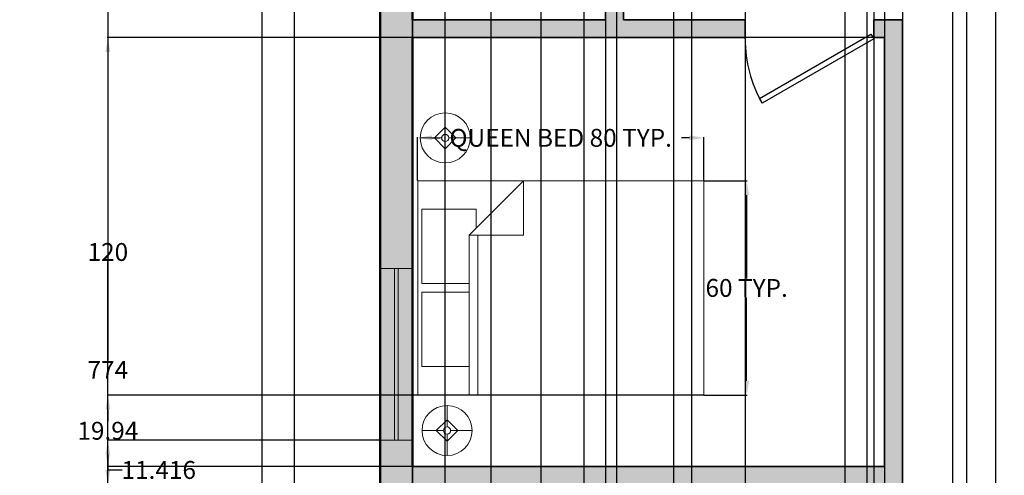
# Model space of a CAD drawing. Units: inches. Extents: x 882 to 1363, y 890 to 1847.
# Tile 5 of 9: x 882 to 1157, y 1351 to 1479. Entities that reach past the tile are written whole.
import ezdxf

# ---------------------------------------------------------------- set-up
doc = ezdxf.new("R2010")
doc.units = ezdxf.units.IN
doc.header["$MEASUREMENT"] = 0
for name, color, linetype, lineweight in [('A-ANNO-DIMS', 2, 'Continuous', 18), ('C-PROP', 7, 'Continuous', 25), ('doors', 3, 'Continuous', 25), ('furniture', 10, 'Continuous', 18), ('inner wall', 50, 'Continuous', 35), ('outer wall', 40, 'Continuous', 50), ('windows', 226, 'Continuous', 18)]:
    doc.layers.add(name, color=color, linetype=linetype, lineweight=lineweight)
doc.layers.add('A-WALL-PATT', color=251, linetype='Continuous', lineweight=13, true_color=0x636466)
doc.styles.get("Standard").update_dxf_attribs({"font": 'arial.ttf'})
doc.dimstyles.get("Standard").update_dxf_attribs({"dimtxt": 5, "dimasz": 4, "dimexe": 0.18, "dimexo": 0.0625, "dimgap": 0.09, "dimtad": 0, "dimtih": 1, "dimtoh": 1, "dimdec": 1, "dimzin": 0, "dimdsep": 46, "dimlunit": 3, "dimtxsty": 'Standard', "dimcen": 0.09, "dimadec": 0, "dimazin": 0, "dimtfac": 1, "dimtdec": 1, "dimtofl": 0, "dimtmove": 0, "dimatfit": 3, "dimfxl": 1, "dimtolj": 1, "dimtzin": 0, "dimarcsym": 0})

# ---------------------------------------------------------------- blocks, each defined once
blk = doc.blocks.new('*U2')
for p, q in [((0, 0), (0, -6)), ((40, 0), (40, -6))]:
    blk.add_line(p, q)
blk.add_lwpolyline([(0, 0), (34.64, 20), (35.52, 18.48), (0.87, -1.52)], close=True)
blk.add_arc((0, 0), 40, 0, 30)
blk = doc.blocks.new('Bed - Queen')
for p, q in [((0, -80.00003), (0, 0)), ((0, 0), (59.99999, 0)), ((59.99999, 0), (59.99999, -80.00003)), ((7.99999, -1.2), (28.79998, -1.2)), ((7.99999, -14.4), (7.99999, -1.2)), ((28.79998, -1.2), (28.79998, -14.4)), ((31.19999, -1.2), (51.99999, -1.2)), ((31.19999, -14.4), (31.19999, -1.2)), ((51.99999, -1.2), (51.99999, -16.4)), ((0, -14.4), (44.8, -14.4)), ((59.99999, -29.6), (44.8, -14.4)), ((44.8, -14.4), (44.8, -29.6)), ((51.99999, -16.4), (46.79936, -16.4)), ((44.8, -16.8), (0, -16.8)), ((44.8, -29.6), (59.99999, -29.6)), ((59.99999, -80.00003), (0, -80.00003))]:
    blk.add_line(p, q)
blk = doc.blocks.new('Lamp - Table')
for p, q in [((0, 7), (0, 1)), ((0, 3), (-3, 0)), ((3, 0), (0, 3)), ((-1, 0), (-7, 0)), ((-3, 0), (0, -3)), ((0, -3), (3, 0)), ((1, 0), (7, 0)), ((0, -1), (0, -7))]:
    blk.add_line(p, q)
for radius in [7, 1]:
    blk.add_circle((0, 0), radius)
blk = doc.blocks.new('WIN-48IN-9IN')
for p, q in [((4, 0), (4, 48)), ((5, 0), (5, 48))]:
    blk.add_line(p, q)
blk.add_lwpolyline([(0, 48), (9, 48), (9, 0), (0, 0)], close=True)
blk = doc.blocks.new('*D23')
at = {"layer": 'A-ANNO-DIMS', "color": 0, "lineweight": -2, "transparency": 16777216}
for p, q in [((993.28, 1433.75), (993.28, 1445.87)), ((997.28, 1445.69), (999.49, 1445.69)), ((1069.28, 1445.69), (1067.08, 1445.69)), ((1073.28, 1433.75), (1073.28, 1445.87))]:
    blk.add_line(p, q, dxfattribs=at)
at = {"layer": 'A-ANNO-DIMS', "color": 0, "transparency": 16777216}
for points in [[(997.28, 1446.35), (997.28, 1445.02), (993.28, 1445.69)], [(1069.28, 1446.35), (1069.28, 1445.02), (1073.28, 1445.69)]]:
    blk.add_solid(points, dxfattribs=at)
at = {"layer": 'Defpoints', "color": 0, "transparency": 16777216}
for p in [(993.28, 1445.69), (993.28, 1433.69), (1073.28, 1433.69)]:
    blk.add_point(p, dxfattribs=at)
at = {"layer": 'A-ANNO-DIMS', "color": 0, "transparency": 16777216, "insert": (1033.28, 1445.69), "char_height": 5, "attachment_point": 5}
blk.add_mtext('\\A1;QUEEN BED 80 TYP.', dxfattribs=at)
blk = doc.blocks.new('*D24')
at = {"layer": 'A-ANNO-DIMS', "color": 0, "lineweight": -2, "transparency": 16777216}
for p, q in [((1073.34, 1433.69), (1085.46, 1433.69)), ((1085.28, 1429.69), (1085.28, 1406.33)), ((1085.28, 1377.69), (1085.28, 1401.04)), ((1073.34, 1373.69), (1085.46, 1373.69))]:
    blk.add_line(p, q, dxfattribs=at)
at = {"layer": 'A-ANNO-DIMS', "color": 0, "transparency": 16777216}
for points in [[(1084.61, 1429.69), (1085.95, 1429.69), (1085.28, 1433.69)], [(1084.61, 1377.69), (1085.95, 1377.69), (1085.28, 1373.69)]]:
    blk.add_solid(points, dxfattribs=at)
at = {"layer": 'Defpoints', "color": 0, "transparency": 16777216}
for p in [(1073.28, 1433.69), (1085.28, 1433.69), (1073.28, 1373.69)]:
    blk.add_point(p, dxfattribs=at)
at = {"layer": 'A-ANNO-DIMS', "color": 0, "transparency": 16777216, "insert": (1085.28, 1403.69), "char_height": 5, "attachment_point": 5}
blk.add_mtext('\\A1;60 TYP.', dxfattribs=at)
blk = doc.blocks.new('*D37')
at = {"layer": 'A-ANNO-DIMS', "color": 0, "lineweight": -2, "transparency": 16777216}
for p, q in [((982.78, 1767.75), (906.46, 1767.75)), ((906.64, 1763.75), (906.64, 1383.34)), ((906.64, 997.75), (906.64, 1378.16)), ((982.78, 993.75), (906.46, 993.75))]:
    blk.add_line(p, q, dxfattribs=at)
at = {"layer": 'A-ANNO-DIMS', "color": 0, "transparency": 16777216}
for points in [[(905.97, 1763.75), (907.3, 1763.75), (906.64, 1767.75)], [(905.97, 997.75), (907.3, 997.75), (906.64, 993.75)]]:
    blk.add_solid(points, dxfattribs=at)
at = {"layer": 'Defpoints', "color": 0, "transparency": 16777216}
for p in [(906.64, 1767.75), (982.84, 1767.75), (982.84, 993.75)]:
    blk.add_point(p, dxfattribs=at)
at = {"layer": 'A-ANNO-DIMS', "color": 0, "transparency": 16777216, "insert": (906.64, 1380.75), "char_height": 5, "attachment_point": 5}
blk.add_mtext('\\A1;774', dxfattribs=at)
blk = doc.blocks.new('*D40')
at = {"layer": 'A-ANNO-DIMS', "color": 0, "lineweight": -2, "transparency": 16777216}
for p, q in [((991.84, 1758.69), (991.84, 893.37)), ((1064.84, 1758.69), (1064.84, 893.37)), ((995.84, 893.55), (1024.69, 893.55)), ((1060.84, 893.55), (1031.99, 893.55))]:
    blk.add_line(p, q, dxfattribs=at)
at = {"layer": 'A-ANNO-DIMS', "color": 0, "transparency": 16777216}
for points in [[(995.84, 894.21), (995.84, 892.88), (991.84, 893.55)], [(1060.84, 894.21), (1060.84, 892.88), (1064.84, 893.55)]]:
    blk.add_solid(points, dxfattribs=at)
at = {"layer": 'Defpoints', "color": 0, "transparency": 16777216}
for p in [(991.84, 1758.75), (1064.84, 1758.75), (1064.84, 893.55)]:
    blk.add_point(p, dxfattribs=at)
at = {"layer": 'A-ANNO-DIMS', "color": 0, "transparency": 16777216, "insert": (1028.34, 893.55), "char_height": 5, "attachment_point": 5}
blk.add_mtext('\\A1;73', dxfattribs=at)
blk = doc.blocks.new('*D41')
at = {"layer": 'A-ANNO-DIMS', "color": 0, "lineweight": -2, "transparency": 16777216}
for p, q in [((1069.84, 1758.69), (1069.84, 893.37)), ((1154.84, 1758.69), (1154.84, 893.37)), ((1073.84, 893.55), (1108.65, 893.55)), ((1150.84, 893.55), (1116.03, 893.55))]:
    blk.add_line(p, q, dxfattribs=at)
at = {"layer": 'A-ANNO-DIMS', "color": 0, "transparency": 16777216}
for points in [[(1073.84, 894.21), (1073.84, 892.88), (1069.84, 893.55)], [(1150.84, 894.21), (1150.84, 892.88), (1154.84, 893.55)]]:
    blk.add_solid(points, dxfattribs=at)
at = {"layer": 'Defpoints', "color": 0, "transparency": 16777216}
for p in [(1069.84, 1758.75), (1154.84, 1758.75), (1154.84, 893.55)]:
    blk.add_point(p, dxfattribs=at)
at = {"layer": 'A-ANNO-DIMS', "color": 0, "transparency": 16777216, "insert": (1112.34, 893.55), "char_height": 5, "attachment_point": 5}
blk.add_mtext('\\A1;85', dxfattribs=at)
blk = doc.blocks.new('*D47')
at = {"layer": 'A-ANNO-DIMS', "color": 0, "lineweight": -2, "transparency": 16777216}
for p, q in [((1123.84, 1567.69), (1123.84, 893.37)), ((1128.84, 1567.69), (1128.84, 893.37)), ((1119.84, 893.55), (1115.84, 893.55)), ((1132.84, 893.55), (1136.84, 893.55))]:
    blk.add_line(p, q, dxfattribs=at)
at = {"layer": 'A-ANNO-DIMS', "color": 0, "transparency": 16777216}
for points in [[(1119.84, 894.21), (1119.84, 892.88), (1123.84, 893.55)], [(1132.84, 894.21), (1132.84, 892.88), (1128.84, 893.55)]]:
    blk.add_solid(points, dxfattribs=at)
at = {"layer": 'Defpoints', "color": 0, "transparency": 16777216}
for p in [(1123.84, 1567.75), (1128.84, 1567.75), (1128.84, 893.55)]:
    blk.add_point(p, dxfattribs=at)
at = {"layer": 'A-ANNO-DIMS', "color": 0, "transparency": 16777216, "insert": (1126.34, 893.55), "char_height": 5, "attachment_point": 5}
blk.add_mtext('\\A1;5', dxfattribs=at)
blk = doc.blocks.new('*D48')
at = {"layer": 'A-ANNO-DIMS', "color": 0, "lineweight": -2, "transparency": 16777216}
for p, q in [((1084.84, 1562.69), (1084.84, 893.37)), ((1120.84, 1562.69), (1120.84, 893.37)), ((1088.84, 893.55), (1099.17, 893.55)), ((1116.84, 893.55), (1106.51, 893.55))]:
    blk.add_line(p, q, dxfattribs=at)
at = {"layer": 'A-ANNO-DIMS', "color": 0, "transparency": 16777216}
for points in [[(1088.84, 894.21), (1088.84, 892.88), (1084.84, 893.55)], [(1116.84, 894.21), (1116.84, 892.88), (1120.84, 893.55)]]:
    blk.add_solid(points, dxfattribs=at)
at = {"layer": 'Defpoints', "color": 0, "transparency": 16777216}
for p in [(1084.84, 1562.75), (1120.84, 1562.75), (1120.84, 893.55)]:
    blk.add_point(p, dxfattribs=at)
at = {"layer": 'A-ANNO-DIMS', "color": 0, "transparency": 16777216, "insert": (1102.84, 893.55), "char_height": 5, "attachment_point": 5}
blk.add_mtext('\\A1;36', dxfattribs=at)
blk = doc.blocks.new('*D51')
at = {"layer": 'A-ANNO-DIMS', "color": 0, "lineweight": -2, "transparency": 16777216}
for p, q in [((982.84, 1767.69), (982.84, 893.37)), ((1000.84, 1767.69), (1000.84, 893.37)), ((986.84, 893.55), (996.84, 893.55)), ((1000.84, 893.55), (1004.84, 893.55))]:
    blk.add_line(p, q, dxfattribs=at)
at = {"layer": 'A-ANNO-DIMS', "color": 0, "transparency": 16777216}
for points in [[(986.84, 894.21), (986.84, 892.88), (982.84, 893.55)], [(996.84, 894.21), (996.84, 892.88), (1000.84, 893.55)]]:
    blk.add_solid(points, dxfattribs=at)
at = {"layer": 'Defpoints', "color": 0, "transparency": 16777216}
for p in [(982.84, 1767.75), (1000.84, 1767.75), (1000.84, 893.55)]:
    blk.add_point(p, dxfattribs=at)
at = {"layer": 'A-ANNO-DIMS', "color": 0, "transparency": 16777216, "insert": (1015.08, 893.55), "char_height": 5, "attachment_point": 5}
blk.add_mtext('\\A1;18.006', dxfattribs=at)
blk = doc.blocks.new('*D52')
at = {"layer": 'A-ANNO-DIMS', "color": 0, "lineweight": -2, "transparency": 16777216}
for p, q in [((1048.84, 1767.69), (1048.84, 893.37)), ((1118.86, 1767.69), (1118.86, 893.37)), ((1052.84, 893.55), (1075.83, 893.55)), ((1114.86, 893.55), (1091.87, 893.55))]:
    blk.add_line(p, q, dxfattribs=at)
at = {"layer": 'A-ANNO-DIMS', "color": 0, "transparency": 16777216}
for points in [[(1052.84, 894.21), (1052.84, 892.88), (1048.84, 893.55)], [(1114.86, 894.21), (1114.86, 892.88), (1118.86, 893.55)]]:
    blk.add_solid(points, dxfattribs=at)
at = {"layer": 'Defpoints', "color": 0, "transparency": 16777216}
for p in [(1048.84, 1767.75), (1118.86, 1767.75), (1118.86, 893.55)]:
    blk.add_point(p, dxfattribs=at)
at = {"layer": 'A-ANNO-DIMS', "color": 0, "transparency": 16777216, "insert": (1083.85, 893.55), "char_height": 5, "attachment_point": 5}
blk.add_mtext('\\A1;70.01', dxfattribs=at)
blk = doc.blocks.new('*D53')
at = {"layer": 'A-ANNO-DIMS', "color": 0, "lineweight": -2, "transparency": 16777216}
for p, q in [((1142.86, 1767.69), (1142.86, 893.37)), ((1171.41, 1767.69), (1171.41, 893.37)), ((1138.86, 893.55), (1134.86, 893.55)), ((1175.41, 893.55), (1179.41, 893.55))]:
    blk.add_line(p, q, dxfattribs=at)
at = {"layer": 'A-ANNO-DIMS', "color": 0, "transparency": 16777216}
for points in [[(1138.86, 894.21), (1138.86, 892.88), (1142.86, 893.55)], [(1175.41, 894.21), (1175.41, 892.88), (1171.41, 893.55)]]:
    blk.add_solid(points, dxfattribs=at)
at = {"layer": 'Defpoints', "color": 0, "transparency": 16777216}
for p in [(1142.86, 1767.75), (1171.41, 1767.75), (1171.41, 893.55)]:
    blk.add_point(p, dxfattribs=at)
at = {"layer": 'A-ANNO-DIMS', "color": 0, "transparency": 16777216, "insert": (1157.14, 893.55), "char_height": 5, "attachment_point": 5}
blk.add_mtext('\\A1;28.554', dxfattribs=at)
blk = doc.blocks.new('*D58')
at = {"layer": 'A-ANNO-DIMS', "color": 0, "lineweight": -2, "transparency": 16777216}
for p, q in [((1123.78, 1473.75), (906.46, 1473.75)), ((906.64, 1469.75), (906.64, 1416.39)), ((906.64, 1357.75), (906.64, 1411.11)), ((1123.78, 1353.75), (906.46, 1353.75))]:
    blk.add_line(p, q, dxfattribs=at)
at = {"layer": 'A-ANNO-DIMS', "color": 0, "transparency": 16777216}
for points in [[(905.97, 1469.75), (907.3, 1469.75), (906.64, 1473.75)], [(905.97, 1357.75), (907.3, 1357.75), (906.64, 1353.75)]]:
    blk.add_solid(points, dxfattribs=at)
at = {"layer": 'Defpoints', "color": 0, "transparency": 16777216}
for p in [(1123.84, 1473.75), (906.64, 1353.75), (1123.84, 1353.75)]:
    blk.add_point(p, dxfattribs=at)
at = {"layer": 'A-ANNO-DIMS', "color": 0, "transparency": 16777216, "insert": (906.64, 1413.75), "char_height": 5, "attachment_point": 5}
blk.add_mtext('\\A1;120', dxfattribs=at)
blk = doc.blocks.new('*D59')
at = {"layer": 'A-ANNO-DIMS', "color": 0, "lineweight": -2, "transparency": 16777216}
for p, q in [((982.78, 1361.08), (906.46, 1361.08)), ((906.64, 1357.08), (906.64, 1352.75)), ((991.78, 1348.75), (906.46, 1348.75)), ((906.64, 1348.75), (906.64, 1344.75)), ((906.64, 1344.75), (902.64, 1344.75))]:
    blk.add_line(p, q, dxfattribs=at)
at = {"layer": 'A-ANNO-DIMS', "color": 0, "transparency": 16777216}
for points in [[(905.97, 1357.08), (907.3, 1357.08), (906.64, 1361.08)], [(905.97, 1352.75), (907.3, 1352.75), (906.64, 1348.75)]]:
    blk.add_solid(points, dxfattribs=at)
at = {"layer": 'Defpoints', "color": 0, "transparency": 16777216}
for p in [(982.84, 1361.08), (906.64, 1348.75), (991.84, 1348.75)]:
    blk.add_point(p, dxfattribs=at)
at = {"layer": 'A-ANNO-DIMS', "color": 0, "transparency": 16777216, "insert": (892.4, 1344.75), "char_height": 5, "attachment_point": 5}
blk.add_mtext('\\A1;12.328', dxfattribs=at)
blk = doc.blocks.new('*D68')
at = {"layer": 'A-ANNO-DIMS', "color": 0, "lineweight": -2, "transparency": 16777216}
for p, q in [((1027.84, 1142.81), (1027.84, 1844.13)), ((1031.84, 1843.95), (1066.65, 1843.95)), ((1108.84, 1843.95), (1074.03, 1843.95)), ((1112.84, 1142.81), (1112.84, 1844.13))]:
    blk.add_line(p, q, dxfattribs=at)
at = {"layer": 'A-ANNO-DIMS', "color": 0, "transparency": 16777216}
for points in [[(1031.84, 1844.62), (1031.84, 1843.29), (1027.84, 1843.95)], [(1108.84, 1844.62), (1108.84, 1843.29), (1112.84, 1843.95)]]:
    blk.add_solid(points, dxfattribs=at)
at = {"layer": 'Defpoints', "color": 0, "transparency": 16777216}
for p in [(1112.84, 1843.95), (1027.84, 1142.75), (1112.84, 1142.75)]:
    blk.add_point(p, dxfattribs=at)
at = {"layer": 'A-ANNO-DIMS', "color": 0, "transparency": 16777216, "insert": (1070.34, 1843.95), "char_height": 5, "attachment_point": 5}
blk.add_mtext('\\A1;85', dxfattribs=at)
blk = doc.blocks.new('*D74')
at = {"layer": 'A-ANNO-DIMS', "color": 0, "lineweight": -2, "transparency": 16777216}
for p, q in [((991.84, 1002.81), (991.84, 1844.13)), ((995.84, 1843.95), (1012.06, 1843.95)), ((1035.84, 1843.95), (1019.62, 1843.95)), ((1039.84, 1002.81), (1039.84, 1844.13))]:
    blk.add_line(p, q, dxfattribs=at)
at = {"layer": 'A-ANNO-DIMS', "color": 0, "transparency": 16777216}
for points in [[(995.84, 1844.62), (995.84, 1843.29), (991.84, 1843.95)], [(1035.84, 1844.62), (1035.84, 1843.29), (1039.84, 1843.95)]]:
    blk.add_solid(points, dxfattribs=at)
at = {"layer": 'Defpoints', "color": 0, "transparency": 16777216}
for p in [(1039.84, 1843.95), (991.84, 1002.75), (1039.84, 1002.75)]:
    blk.add_point(p, dxfattribs=at)
at = {"layer": 'A-ANNO-DIMS', "color": 0, "transparency": 16777216, "insert": (1015.84, 1843.95), "char_height": 5, "attachment_point": 5}
blk.add_mtext('\\A1;48', dxfattribs=at)
blk = doc.blocks.new('*D78')
at = {"layer": 'A-ANNO-DIMS', "color": 0, "lineweight": -2, "transparency": 16777216}
for p, q in [((1146.84, 1274.81), (1146.84, 1844.13)), ((1150.84, 1843.95), (1179.69, 1843.95)), ((1215.84, 1843.95), (1186.99, 1843.95)), ((1219.84, 1274.81), (1219.84, 1844.13))]:
    blk.add_line(p, q, dxfattribs=at)
at = {"layer": 'A-ANNO-DIMS', "color": 0, "transparency": 16777216}
for points in [[(1150.84, 1844.62), (1150.84, 1843.29), (1146.84, 1843.95)], [(1215.84, 1844.62), (1215.84, 1843.29), (1219.84, 1843.95)]]:
    blk.add_solid(points, dxfattribs=at)
at = {"layer": 'Defpoints', "color": 0, "transparency": 16777216}
for p in [(1219.84, 1843.95), (1146.84, 1274.75), (1219.84, 1274.75)]:
    blk.add_point(p, dxfattribs=at)
at = {"layer": 'A-ANNO-DIMS', "color": 0, "transparency": 16777216, "insert": (1183.34, 1843.95), "char_height": 5, "attachment_point": 5}
blk.add_mtext('\\A1;73', dxfattribs=at)
blk = doc.blocks.new('*D83')
at = {"layer": 'A-ANNO-DIMS', "color": 0, "lineweight": -2, "transparency": 16777216}
for p, q in [((906.64, 1348.75), (906.64, 1352.75)), ((906.64, 1352.75), (910.64, 1352.75)), ((991.78, 1348.75), (906.46, 1348.75)), ((906.64, 1341.33), (906.64, 1344.75)), ((982.78, 1337.33), (906.46, 1337.33))]:
    blk.add_line(p, q, dxfattribs=at)
at = {"layer": 'A-ANNO-DIMS', "color": 0, "transparency": 16777216}
for points in [[(905.97, 1344.75), (907.3, 1344.75), (906.64, 1348.75)], [(905.97, 1341.33), (907.3, 1341.33), (906.64, 1337.33)]]:
    blk.add_solid(points, dxfattribs=at)
at = {"layer": 'Defpoints', "color": 0, "transparency": 16777216}
for p in [(906.64, 1348.75), (991.84, 1348.75), (982.84, 1337.33)]:
    blk.add_point(p, dxfattribs=at)
at = {"layer": 'A-ANNO-DIMS', "color": 0, "transparency": 16777216, "insert": (920.87, 1352.75), "char_height": 5, "attachment_point": 5}
blk.add_mtext('\\A1;11.416', dxfattribs=at)
blk = doc.blocks.new('*D85')
at = {"layer": 'A-ANNO-DIMS', "color": 0, "lineweight": -2, "transparency": 16777216}
for p, q in [((1045.84, 1562.69), (1045.84, 893.37)), ((1084.84, 1562.69), (1084.84, 893.37)), ((1049.84, 893.55), (1061.66, 893.55)), ((1080.84, 893.55), (1069.01, 893.55))]:
    blk.add_line(p, q, dxfattribs=at)
at = {"layer": 'A-ANNO-DIMS', "color": 0, "transparency": 16777216}
for points in [[(1049.84, 894.21), (1049.84, 892.88), (1045.84, 893.55)], [(1080.84, 894.21), (1080.84, 892.88), (1084.84, 893.55)]]:
    blk.add_solid(points, dxfattribs=at)
at = {"layer": 'Defpoints', "color": 0, "transparency": 16777216}
for p in [(1045.84, 1562.75), (1084.84, 1562.75), (1084.84, 893.55)]:
    blk.add_point(p, dxfattribs=at)
at = {"layer": 'A-ANNO-DIMS', "color": 0, "transparency": 16777216, "insert": (1065.34, 893.55), "char_height": 5, "attachment_point": 5}
blk.add_mtext('\\A1;39', dxfattribs=at)
blk = doc.blocks.new('*D88')
at = {"layer": 'A-ANNO-DIMS', "color": 0, "lineweight": -2, "transparency": 16777216}
for p, q in [((1128.84, 1567.69), (1128.84, 893.37)), ((1211.84, 1562.69), (1211.84, 893.37)), ((1132.84, 893.55), (1166.66, 893.55)), ((1207.84, 893.55), (1174.01, 893.55))]:
    blk.add_line(p, q, dxfattribs=at)
at = {"layer": 'A-ANNO-DIMS', "color": 0, "transparency": 16777216}
for points in [[(1132.84, 894.21), (1132.84, 892.88), (1128.84, 893.55)], [(1207.84, 894.21), (1207.84, 892.88), (1211.84, 893.55)]]:
    blk.add_solid(points, dxfattribs=at)
at = {"layer": 'Defpoints', "color": 0, "transparency": 16777216}
for p in [(1128.84, 1567.75), (1211.84, 1562.75), (1211.84, 893.55)]:
    blk.add_point(p, dxfattribs=at)
at = {"layer": 'A-ANNO-DIMS', "color": 0, "transparency": 16777216, "insert": (1170.34, 893.55), "char_height": 5, "attachment_point": 5}
blk.add_mtext('\\A1;83', dxfattribs=at)
blk = doc.blocks.new('*D89')
at = {"layer": 'A-ANNO-DIMS', "color": 0, "lineweight": -2, "transparency": 16777216}
for p, q in [((991.84, 1473.69), (991.84, 893.37)), ((1084.84, 1473.69), (1084.84, 893.37)), ((995.84, 893.55), (1034.67, 893.55)), ((1080.84, 893.55), (1042.01, 893.55))]:
    blk.add_line(p, q, dxfattribs=at)
at = {"layer": 'A-ANNO-DIMS', "color": 0, "transparency": 16777216}
for points in [[(995.84, 894.21), (995.84, 892.88), (991.84, 893.55)], [(1080.84, 894.21), (1080.84, 892.88), (1084.84, 893.55)]]:
    blk.add_solid(points, dxfattribs=at)
at = {"layer": 'Defpoints', "color": 0, "transparency": 16777216}
for p in [(991.84, 1473.75), (1084.84, 1473.75), (1084.84, 893.55)]:
    blk.add_point(p, dxfattribs=at)
at = {"layer": 'A-ANNO-DIMS', "color": 0, "transparency": 16777216, "insert": (1038.34, 893.55), "char_height": 5, "attachment_point": 5}
blk.add_mtext('\\A1;93', dxfattribs=at)
blk = doc.blocks.new('*D92')
at = {"layer": 'A-ANNO-DIMS', "color": 0, "lineweight": -2, "transparency": 16777216}
for p, q in [((1073.22, 1373.69), (906.46, 1373.69)), ((906.64, 1369.69), (906.64, 1366.36)), ((906.64, 1357.75), (906.64, 1361.08)), ((1123.78, 1353.75), (906.46, 1353.75))]:
    blk.add_line(p, q, dxfattribs=at)
at = {"layer": 'A-ANNO-DIMS', "color": 0, "transparency": 16777216}
for points in [[(905.97, 1369.69), (907.3, 1369.69), (906.64, 1373.69)], [(905.97, 1357.75), (907.3, 1357.75), (906.64, 1353.75)]]:
    blk.add_solid(points, dxfattribs=at)
at = {"layer": 'Defpoints', "color": 0, "transparency": 16777216}
for p in [(1073.28, 1373.69), (906.64, 1353.75), (1123.84, 1353.75)]:
    blk.add_point(p, dxfattribs=at)
at = {"layer": 'A-ANNO-DIMS', "color": 0, "transparency": 16777216, "insert": (906.64, 1363.72), "char_height": 5, "attachment_point": 5}
blk.add_mtext('\\A1;19.94', dxfattribs=at)
blk = doc.blocks.new('*D93')
at = {"layer": 'A-ANNO-DIMS', "color": 0, "lineweight": -2, "transparency": 16777216}
for p, q in [((987.84, 1843.95), (983.84, 1843.95)), ((991.84, 1337.4), (991.84, 1844.13)), ((1013.79, 1306.45), (1013.79, 1844.13)), ((1017.79, 1843.95), (1021.79, 1843.95))]:
    blk.add_line(p, q, dxfattribs=at)
at = {"layer": 'A-ANNO-DIMS', "color": 0, "transparency": 16777216}
for points in [[(987.84, 1844.62), (987.84, 1843.29), (991.84, 1843.95)], [(1017.79, 1844.62), (1017.79, 1843.29), (1013.79, 1843.95)]]:
    blk.add_solid(points, dxfattribs=at)
at = {"layer": 'Defpoints', "color": 0, "transparency": 16777216}
for p in [(1013.79, 1843.95), (991.84, 1337.33), (1013.79, 1306.39)]:
    blk.add_point(p, dxfattribs=at)
at = {"layer": 'A-ANNO-DIMS', "color": 0, "transparency": 16777216, "insert": (1002.81, 1843.95), "char_height": 5, "attachment_point": 5}
blk.add_mtext('\\A1;21.95', dxfattribs=at)

msp = doc.modelspace()

# ---------------------------------------------------------------- hatches: boundary and pattern name
at = {"layer": 'A-WALL-PATT'}
h = msp.add_hatch(color=256, dxfattribs=at)
h.dxf.hatch_style = 1
h.paths.add_polyline_path([(1050.8388, 1481.7495), (1050.8388, 1478.7495), (1084.8388, 1478.7495), (1084.8388, 1473.7495), (991.8388, 1473.7495), (991.8388, 1361.0778), (982.8388, 1361.0778), (982.8388, 1556.1531), (991.8388, 1556.1531), (991.8388, 1478.7495), (1045.8388, 1478.7495), (1045.8388, 1481.7479), (1045.4161, 1481.7477), (1030.9055, 1506.8563), (1032.004, 1507.4911), (1046.5146, 1482.3825), (1045.4161, 1481.7477), (1045.8388, 1481.7479), (1045.8388, 1481.7495)])
h.paths.add_polyline_path([(1128.8388, 1478.7495), (1120.8388, 1478.7495), (1120.8388, 1473.7495), (1123.8388, 1473.7495), (1123.8388, 1353.7495), (991.8388, 1353.7495), (991.8388, 1361.0778), (982.8388, 1361.0778), (982.8388, 1337.3333), (991.8388, 1337.3333), (991.8388, 1348.7495), (1128.8388, 1348.7495)])
h.paths.add_polyline_path([(1118.8585, 1767.7495), (1048.8447, 1767.7495), (1048.8447, 1758.7495), (1064.8388, 1758.7495), (1069.8388, 1758.7495), (1118.8585, 1758.7495)])
h.paths.add_polyline_path([(1171.4129, 1767.7495), (1142.8585, 1767.7495), (1142.8585, 1758.7495), (1154.8388, 1758.7495), (1154.8388, 1710.7495), (1069.8388, 1710.7495), (1069.8388, 1713.7495), (1064.8388, 1713.7495), (1064.8388, 1705.7495), (1123.8388, 1705.7495), (1123.8388, 1567.7495), (1120.8388, 1567.7495), (1120.8388, 1562.7495), (1123.8388, 1562.7495), (1211.8388, 1562.7495), (1211.8388, 1567.7495), (1128.8388, 1567.7495), (1128.8388, 1705.7495), (1211.8388, 1705.7495), (1211.8388, 1710.7495), (1159.8388, 1710.7495), (1159.8388, 1758.7495), (1171.4129, 1758.7495)])
h.paths.add_polyline_path([(1252.8388, 1767.7495), (1195.4129, 1767.7495), (1195.4129, 1758.7495), (1243.8388, 1758.7495), (1243.8388, 1710.7495), (1240.8388, 1710.7495), (1240.8388, 1706.4648), (1240.8388, 1705.7495), (1243.8388, 1705.7495), (1243.8388, 1673.1735), (1252.8388, 1673.1735)])
h.paths.add_polyline_path([(1252.8388, 1625.1735), (1243.8388, 1625.1735), (1243.8388, 1567.7495), (1240.8388, 1567.7495), (1240.8388, 1562.7495), (1243.8388, 1562.7495), (1243.8388, 1546.029), (1252.8388, 1546.029)])
h.paths.add_polyline_path([(1252.8388, 1498.029), (1243.8388, 1498.029), (1243.8388, 1391.1399), (1252.8388, 1391.1399)])
h.paths.add_polyline_path([(1252.8388, 1179.8561), (1243.8388, 1179.8561), (1243.8388, 1149.7495), (1219.8388, 1149.7495), (1219.8388, 1145.3111), (1219.8388, 1144.7495), (1252.8388, 1144.7495)])
h.paths.add_polyline_path([(1252.8388, 1277.7495), (1243.8388, 1277.7495), (1243.8388, 1274.7495), (1219.8388, 1274.7495), (1219.8388, 1269.7495), (1243.8388, 1269.7495), (1243.8388, 1227.8561), (1252.8388, 1227.8561)])
h.paths.add_polyline_path([(1252.8388, 1343.1399), (1243.8388, 1343.1399), (1243.8388, 1313.7495), (1248.3388, 1313.7495), (1252.8388, 1313.7495)])
h.paths.add_polyline_path([(1146.8388, 1274.7495), (1112.8388, 1274.7495), (1112.8388, 1106.7495), (1106.7761, 1106.7495), (1106.7761, 1101.7495), (1117.8388, 1101.7495), (1117.8388, 1144.7495), (1159.8388, 1144.7495), (1159.8388, 1149.7495), (1117.8388, 1149.7495), (1117.8388, 1269.7495), (1146.8388, 1269.7495)])

# ---------------------------------------------------------------- linework, layer by layer
at = {"layer": 'C-PROP'}
for points in [[(949.8388, 1800.7495), (1309.8388, 1800.7495), (1309.8388, 936.7495), (949.8388, 936.7495)], [(958.8388, 1791.7495), (1300.8388, 1791.7495), (1300.8388, 945.7495), (958.8388, 945.7495)]]:
    msp.add_lwpolyline(points, close=True, dxfattribs=at)
at = {"layer": 'inner wall'}
for p, q in [((1045.8388, 1478.7495), (1045.8388, 1481.7495)), ((1050.8388, 1478.7495), (1050.8388, 1481.7495)), ((991.8388, 1478.7495), (1045.8388, 1478.7495)), ((1050.8388, 1478.7495), (1084.8388, 1478.7495)), ((1084.8388, 1473.7495), (1084.8388, 1478.7495)), ((1120.8388, 1473.7495), (1120.8388, 1478.7495)), ((1120.8388, 1478.7495), (1128.8388, 1478.7495)), ((1128.8388, 1348.7495), (1128.8388, 1478.7495)), ((991.8388, 1473.7495), (1084.8388, 1473.7495)), ((1120.8388, 1473.7495), (1123.8388, 1473.7495)), ((1123.8388, 1353.7495), (1123.8388, 1473.7495)), ((991.8388, 1353.7495), (1123.8388, 1353.7495))]:
    msp.add_line(p, q, dxfattribs=at)
at = {"layer": 'outer wall'}
for p, q in [((982.8388, 993.7495), (982.8388, 1767.7495)), ((991.8388, 1478.7495), (991.8388, 1562.7495)), ((991.8388, 1353.7495), (991.8388, 1473.7495))]:
    msp.add_line(p, q, dxfattribs=at)

# ---------------------------------------------------------------- block references
at = {"layer": 'doors', "xscale": 0.9, "yscale": 0.9, "zscale": 0.9, "rotation": 180}
msp.add_blockref('*U2', (1120.8388, 1473.3495), dxfattribs=at)
at = {"layer": 'furniture'}
for p in [(1000.9973, 1445.6555), (1001.4971, 1363.7786)]:
    msp.add_blockref('Lamp - Table', p, dxfattribs=at)
at = {"layer": 'furniture', "rotation": 90}
msp.add_blockref('Bed - Queen', (993.2814, 1373.6878), dxfattribs=at)
at = {"layer": 'windows'}
msp.add_blockref('WIN-48IN-9IN', (982.839, 1361.078), dxfattribs=at)

# ---------------------------------------------------------------- dimensions: what is measured, and where the dimension line sits
at = {"layer": 'A-ANNO-DIMS'}
for base, p1, p2, override, picture, middle in [((1013.7874, 1843.953), (991.8388, 1337.3333), (1013.7874, 1306.3919), {"dimdec": 2, "dimlfac": 1, "dimrnd": 0, "dimzin": 0, "dimdsep": 46, "dimlunit": 2}, '*D93', (1002.8131, 1843.953)), ((1039.8388, 1843.953), (991.8388, 1002.7495), (1039.8388, 1002.7495), {"dimdec": 0, "dimlfac": 1, "dimrnd": 0, "dimzin": 0, "dimdsep": 46, "dimlunit": 2}, '*D74', (1015.8388, 1843.953)), ((1112.8388, 1843.953), (1027.8388, 1142.7495), (1112.8388, 1142.7495), {"dimdec": 0, "dimlfac": 1, "dimrnd": 0, "dimzin": 0, "dimdsep": 46, "dimlunit": 2}, '*D68', (1070.3388, 1843.953)), ((1219.8388, 1843.953), (1146.8388, 1274.7495), (1219.8388, 1274.7495), {"dimdec": 0, "dimlfac": 1, "dimrnd": 0, "dimzin": 0, "dimdsep": 46, "dimlunit": 2}, '*D78', (1183.3388, 1843.953)), ((1000.8447, 893.546), (982.8388, 1767.7495), (1000.8447, 1767.7495), {"dimdec": 3, "dimlfac": 1, "dimrnd": 0, "dimzin": 0, "dimdsep": 46, "dimlunit": 2}, '*D51', (1015.0762, 893.546)), ((1118.8585, 893.546), (1048.8447, 1767.7495), (1118.8585, 1767.7495), {"dimdec": 2, "dimlfac": 1, "dimrnd": 0, "dimzin": 0, "dimdsep": 46, "dimlunit": 2}, '*D52', (1083.8516, 893.546)), ((1171.4129, 893.546), (1142.8585, 1767.7495), (1171.4129, 1767.7495), {"dimdec": 3, "dimlfac": 1, "dimrnd": 0, "dimzin": 0, "dimdsep": 46, "dimlunit": 2}, '*D53', (1157.1357, 893.546)), ((1064.8388, 893.546), (991.8388, 1758.7495), (1064.8388, 1758.7495), {"dimdec": 0, "dimlfac": 1, "dimrnd": 0, "dimzin": 0, "dimdsep": 46, "dimlunit": 2}, '*D40', (1028.3388, 893.546)), ((1154.8388, 893.546), (1069.8388, 1758.7495), (1154.8388, 1758.7495), {"dimdec": 0, "dimlfac": 1, "dimrnd": 0, "dimzin": 0, "dimdsep": 46, "dimlunit": 2}, '*D41', (1112.3388, 893.546)), ((1128.8388, 893.546), (1123.8388, 1567.7495), (1128.8388, 1567.7495), {"dimdec": 0, "dimlfac": 1, "dimrnd": 0, "dimzin": 0, "dimdsep": 46, "dimlunit": 2}, '*D47', (1126.3388, 893.546)), ((1211.8388, 893.546), (1128.8388, 1567.7495), (1211.8388, 1562.7495), {"dimdec": 0, "dimlfac": 1, "dimrnd": 0, "dimzin": 0, "dimdsep": 46, "dimlunit": 2}, '*D88', (1170.3388, 893.546)), ((1084.8388, 893.546), (1045.8388, 1562.7495), (1084.8388, 1562.7495), {"dimdec": 0, "dimlfac": 1, "dimrnd": 0, "dimzin": 0, "dimdsep": 46, "dimlunit": 2}, '*D85', (1065.3388, 893.546)), ((1120.8388, 893.546), (1084.8388, 1562.7495), (1120.8388, 1562.7495), {"dimdec": 0, "dimlfac": 1, "dimrnd": 0, "dimzin": 0, "dimdsep": 46, "dimlunit": 2}, '*D48', (1102.8388, 893.546)), ((1084.8388, 893.546), (991.8388, 1473.7495), (1084.8388, 1473.7495), {"dimdec": 0, "dimlfac": 1, "dimrnd": 0, "dimzin": 0, "dimdsep": 46, "dimlunit": 2}, '*D89', (1038.3388, 893.546))]:
    dim = msp.add_linear_dim(base=base, p1=p1, p2=p2, dimstyle='Standard', override=override, dxfattribs=at)
    dim.commit()
    dim.dimension.update_dxf_attribs({"geometry": picture, "text_midpoint": middle})
for base, p1, p2, override, picture, middle in [((906.6353, 1767.7495), (982.8388, 993.7495), (982.8388, 1767.7495), {"dimdec": 0, "dimlfac": 1, "dimrnd": 0, "dimzin": 0, "dimdsep": 46, "dimlunit": 2}, '*D37', (906.6353, 1380.7495)), ((906.6353, 1353.7495), (1123.8388, 1473.7495), (1123.8388, 1353.7495), {"dimdec": 0, "dimlfac": 1, "dimrnd": 0, "dimzin": 0, "dimdsep": 46, "dimlunit": 2}, '*D58', (906.6353, 1413.7495)), ((906.6353, 1353.7495), (1073.2814, 1373.6878), (1123.8388, 1353.7495), {"dimdec": 2, "dimlfac": 1, "dimrnd": 0, "dimzin": 0, "dimdsep": 46, "dimlunit": 2}, '*D92', (906.6353, 1363.7187)), ((906.6353, 1348.7495), (982.8388, 1361.0778), (991.8388, 1348.7495), {"dimdec": 3, "dimlfac": 1, "dimrnd": 0, "dimzin": 0, "dimdsep": 46, "dimlunit": 2}, '*D59', (892.397, 1344.7495)), ((906.6353, 1348.7495), (982.8388, 1337.3333), (991.8388, 1348.7495), {"dimdec": 3, "dimlfac": 1, "dimrnd": 0, "dimzin": 0, "dimdsep": 46, "dimlunit": 2}, '*D83', (920.8669, 1352.7495))]:
    dim = msp.add_linear_dim(base=base, p1=p1, p2=p2, angle=90, dimstyle='Standard', override=override, dxfattribs=at)
    dim.commit()
    dim.dimension.update_dxf_attribs({"geometry": picture, "text_midpoint": middle})
for base, p1, p2, angle, text, picture, middle in [((993.2814, 1445.6878), (1073.2814, 1433.6878), (993.2814, 1433.6878), 180, 'QUEEN BED <> TYP.', '*D23', (1033.2814, 1445.6878)), ((1085.2814, 1433.6878), (1073.2814, 1373.6878), (1073.2814, 1433.6878), 90, '<> TYP.', '*D24', (1085.2814, 1403.6878))]:
    dim = msp.add_linear_dim(base=base, p1=p1, p2=p2, angle=angle, text=text, dimstyle='Standard', override={"dimdec": 0, "dimlfac": 1, "dimrnd": 0, "dimzin": 0, "dimdsep": 46, "dimlunit": 2}, dxfattribs=at)
    dim.commit()
    dim.dimension.update_dxf_attribs({"geometry": picture, "text_midpoint": middle})

doc.saveas('drawing.dxf')
